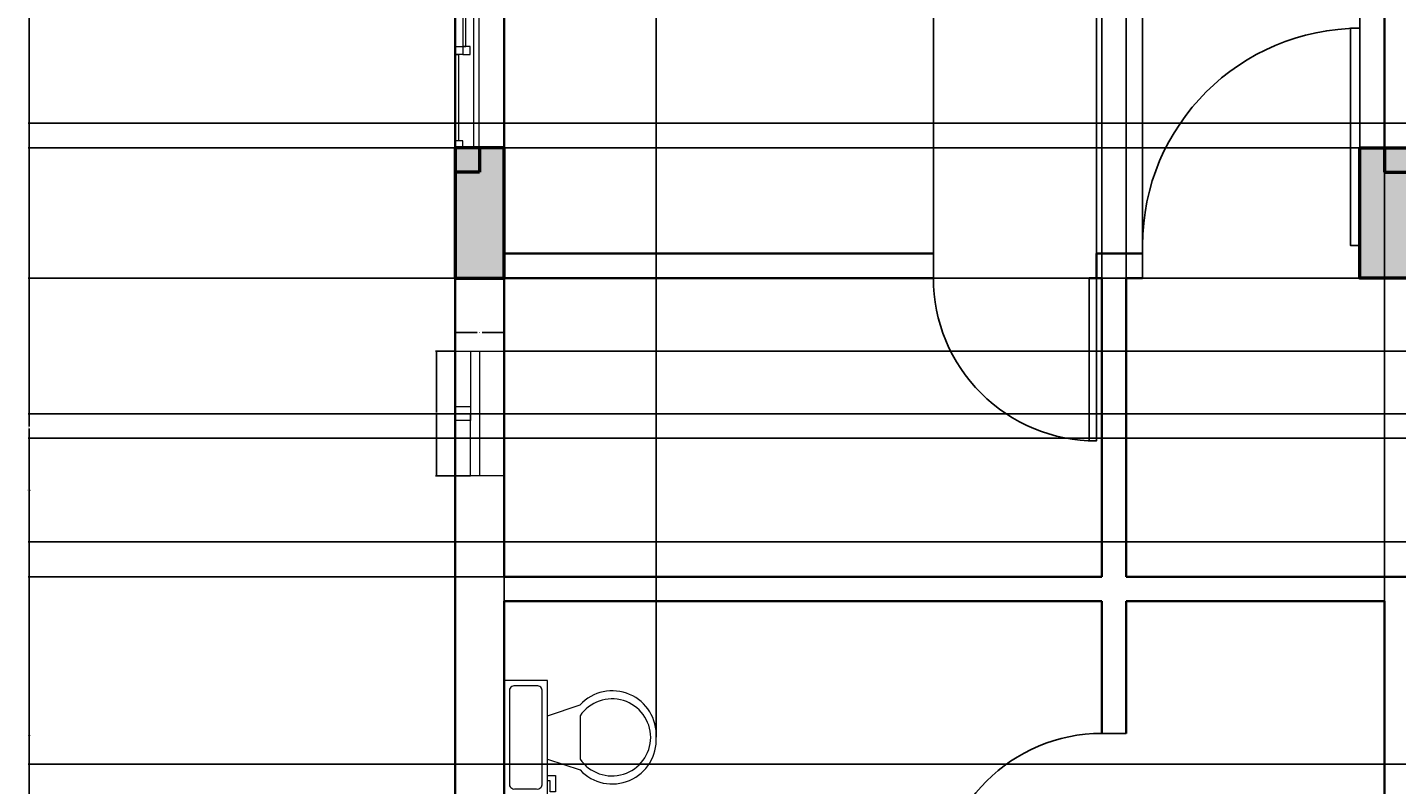
# Model space of a CAD drawing. Units: inches. Extents: x 393 to 993, y 153 to 660.
# Tile 2 of 6: x 393 to 645, y 359 to 499. Entities that reach past the tile are written whole.
import ezdxf

# ---------------------------------------------------------------- set-up
doc = ezdxf.new("R2010")
doc.units = ezdxf.units.IN
doc.header["$MEASUREMENT"] = 0
for name, color, linetype, lineweight in [('A-ANNO-DIMS', 2, 'Continuous', 18), ('A-COLS', 40, 'Continuous', 50), ('A-FLOR-FIXT', 9, 'Continuous', 18), ('A-GLAZ', 4, 'Continuous', 20), ('A-WALL', 40, 'Continuous', 35), ('DOORS', 32, 'Continuous', 25)]:
    doc.layers.add(name, color=color, linetype=linetype, lineweight=lineweight)
doc.styles.get("Standard").update_dxf_attribs({"font": 'arial.ttf'})
doc.dimstyles.get("Standard").update_dxf_attribs({"dimtxt": 0.18, "dimasz": 0.18, "dimexe": 0.18, "dimexo": 0.0625, "dimgap": 0.09, "dimtad": 0, "dimtih": 1, "dimtoh": 1, "dimdec": 1, "dimzin": 0, "dimdsep": 46, "dimlunit": 3, "dimtxsty": 'Standard', "dimcen": 0.09, "dimadec": 0, "dimazin": 0, "dimtfac": 1, "dimtdec": 1, "dimtofl": 0, "dimtmove": 0, "dimatfit": 3, "dimfxl": 1, "dimtolj": 1, "dimtzin": 0, "dimarcsym": 0})

# ---------------------------------------------------------------- blocks, each defined once
blk = doc.blocks.new('W')
for p, q in [((518.15, 606.48), (554.15, 606.48)), ((518.15, 605.48), (554.15, 605.48))]:
    blk.add_line(p, q)
for points in [[(518.15, 609.91), (554.15, 609.91), (554.15, 600.91), (518.15, 600.91)], [(519.42, 609.91), (518.15, 609.91), (518.15, 608.51), (519.42, 608.51)], [(519.42, 609.91), (535.35, 609.91), (535.35, 609.3), (519.42, 609.3)], [(535.35, 609.91), (536.78, 609.91), (536.78, 608.51), (535.35, 608.51)], [(536.78, 608.51), (535.35, 608.51), (535.35, 607.12), (536.78, 607.12)], [(552.72, 608.51), (536.78, 608.51), (536.78, 607.91), (552.72, 607.91)], [(552.72, 608.51), (554.15, 608.51), (554.15, 607.12), (552.72, 607.12)]]:
    blk.add_lwpolyline(points, close=True)
blk = doc.blocks.new('*U3')
for p, q in [((0, 0), (0, -6)), ((40, 0), (40, -6))]:
    blk.add_line(p, q)
blk.add_lwpolyline([(0, 0), (0, 40), (1.75, 40), (1.75, 0)], close=True)
blk.add_arc((0, 0), 40, 0, 90)
blk = doc.blocks.new('MM')
blk.add_line((476.48, 438.96), (476.48, 415.96))
for points in [[(471.98, 438.96), (480.98, 438.96), (480.98, 415.96), (471.98, 415.96), (471.98, 438.96)], [(471.98, 427.46), (471.98, 438.96), (474.84, 438.96), (474.84, 427.46)], [(471.98, 427.46), (471.98, 415.96), (474.84, 415.96), (474.84, 427.46)]]:
    blk.add_lwpolyline(points)
blk.add_lwpolyline([(471.98, 428.78), (474.84, 428.78), (474.84, 426.2), (471.98, 426.2)], close=True)
blk = doc.blocks.new('*U11')
for p, q in [((9.5, -6), (9.5, -2)), ((-10, -8.5), (-8, -8.5)), ((-10, -9.5), (-10, -8.5)), ((-7, -9.5), (-10, -9.5)), ((-8, -8.5), (-8, -8)), ((-7, -8), (-7, -9.5)), ((-4, -8), (-6, -14)), ((4, -8), (6, -14)), ((4, -14), (-4, -14))]:
    blk.add_line(p, q)
blk.add_lwpolyline([(10.5, -8), (10.5, 0), (-10.5, 0), (-10.5, -8)], close=True)
for points in [[(-9.5, -2), (-9.5, -6)], [(8.5, -1), (-8.5, -1)], [(-8.5, -7), (8.5, -7)]]:
    blk.add_lwpolyline(points)
for centre, radius, start, end in [((-8.625, -1.875), 0.8839, 81.8699, 188.1301), ((8.625, -1.875), 0.8839, 351.8699, 98.1301), ((-8.625, -6.125), 0.8839, 171.869898, 278.1301), ((8.625, -6.125), 0.8839, 261.8699, 8.1301), ((-0.4772, -19.9188), 8.0953, 133.01722, 273.38), ((0.0374, -19.8731), 7.127, 124.50543, 269.7), ((-0.0373, -19.8731), 7.127, 270.3, 55.4946), ((0.4773, -19.9188), 8.0953, 266.62, 46.9828)]:
    blk.add_arc(centre, radius, start, end)
blk = doc.blocks.new('COL-9X24-RH')
h = blk.add_hatch(color=256)
h.dxf.hatch_style = 1
h.paths.add_polyline_path([(4.5, 19.5), (4.5, 24), (0, 24), (0, 0), (9, 0), (9, 19.5)])
h = blk.add_hatch(color=256)
h.dxf.hatch_style = 1
h.paths.add_polyline_path([(4.5, 19.5), (9, 19.5), (9, 24), (4.5, 24)])
for p, q in [((4.5, 24), (4.5, 19.5)), ((4.5, 24), (9, 24)), ((9, 24), (9, 19.5)), ((4.5, 19.5), (9, 19.5))]:
    blk.add_line(p, q)
blk.add_lwpolyline([(0, 24), (9, 24), (9, 0), (0, 0), (0, 24)])
blk = doc.blocks.new('COL-9X24-LH')
h = blk.add_hatch(color=256)
h.dxf.hatch_style = 1
h.paths.add_polyline_path([(4.5, 24), (0, 24), (0, 19.5), (4.5, 19.5)])
h = blk.add_hatch(color=256)
h.dxf.hatch_style = 1
h.paths.add_polyline_path([(4.5, 19.5), (0, 19.5), (0, 0), (9, 0), (9, 24), (4.5, 24)])
for p, q in [((4.5, 24), (0, 24)), ((0, 24), (0, 19.5)), ((4.5, 24), (4.5, 19.5)), ((4.5, 19.5), (0, 19.5))]:
    blk.add_line(p, q)
blk.add_lwpolyline([(9, 24), (0, 24), (0, 0), (9, 0), (9, 24)])
blk = doc.blocks.new('*D26')
at = {"layer": 'A-ANNO-DIMS', "color": 0, "lineweight": -2, "transparency": 16777216}
for p, q in [((471.92, 438.96), (468.35, 438.96)), ((468.53, 438.78), (468.53, 427.64)), ((468.53, 416.14), (468.53, 427.27)), ((471.92, 415.96), (468.35, 415.96))]:
    blk.add_line(p, q, dxfattribs=at)
at = {"layer": 'A-ANNO-DIMS', "color": 0, "transparency": 16777216}
for points in [[(468.5, 438.78), (468.56, 438.78), (468.53, 438.96)], [(468.5, 416.14), (468.56, 416.14), (468.53, 415.96)]]:
    blk.add_solid(points, dxfattribs=at)
at = {"layer": 'Defpoints', "color": 0, "transparency": 16777216}
for p in [(468.53, 438.96), (471.98, 438.96), (471.98, 415.96)]:
    blk.add_point(p, dxfattribs=at)
at = {"layer": 'A-ANNO-DIMS', "color": 0, "transparency": 16777216, "insert": (468.53, 427.46), "char_height": 0.18, "attachment_point": 5}
blk.add_mtext('\\A1;WINDOW B 23 TYP.', dxfattribs=at)
blk = doc.blocks.new('*D27')
at = {"layer": 'A-ANNO-DIMS', "color": 0, "lineweight": -2, "transparency": 16777216}
for p, q in [((471.98, 439.02), (471.98, 442.59)), ((472.16, 442.41), (476.02, 442.41)), ((480.8, 442.41), (476.94, 442.41)), ((480.98, 439.02), (480.98, 442.59))]:
    blk.add_line(p, q, dxfattribs=at)
at = {"layer": 'A-ANNO-DIMS', "color": 0, "transparency": 16777216}
for points in [[(472.16, 442.44), (472.16, 442.38), (471.98, 442.41)], [(480.8, 442.44), (480.8, 442.38), (480.98, 442.41)]]:
    blk.add_solid(points, dxfattribs=at)
at = {"layer": 'Defpoints', "color": 0, "transparency": 16777216}
for p in [(480.98, 442.41), (471.98, 438.96), (480.98, 438.96)]:
    blk.add_point(p, dxfattribs=at)
at = {"layer": 'A-ANNO-DIMS', "color": 0, "transparency": 16777216, "insert": (476.48, 442.41), "char_height": 0.18, "attachment_point": 5}
blk.add_mtext('\\A1;9 TYP.', dxfattribs=at)
blk = doc.blocks.new('*D52')
at = {"layer": 'A-ANNO-DIMS', "color": 0, "lineweight": -2, "transparency": 16777216}
for p, q in [((480.92, 397.41), (393.4, 397.41)), ((393.58, 397.23), (393.58, 368.34)), ((393.58, 339.09), (393.58, 367.97)), ((471.92, 338.91), (393.4, 338.91))]:
    blk.add_line(p, q, dxfattribs=at)
at = {"layer": 'A-ANNO-DIMS', "color": 0, "transparency": 16777216}
for points in [[(393.55, 397.23), (393.61, 397.23), (393.58, 397.41)], [(393.55, 339.09), (393.61, 339.09), (393.58, 338.91)]]:
    blk.add_solid(points, dxfattribs=at)
at = {"layer": 'Defpoints', "color": 0, "transparency": 16777216}
for p in [(393.58, 397.41), (480.98, 397.41), (471.98, 338.91)]:
    blk.add_point(p, dxfattribs=at)
at = {"layer": 'A-ANNO-DIMS', "color": 0, "transparency": 16777216, "insert": (393.58, 368.16), "char_height": 0.18, "attachment_point": 5}
blk.add_mtext('\\A1;58.5', dxfattribs=at)
blk = doc.blocks.new('*D53')
at = {"layer": 'A-ANNO-DIMS', "color": 0, "lineweight": -2, "transparency": 16777216}
for p, q in [((471.92, 452.41), (393.4, 452.41)), ((393.58, 452.23), (393.58, 425.09)), ((393.58, 397.59), (393.58, 424.73)), ((480.92, 397.41), (393.4, 397.41))]:
    blk.add_line(p, q, dxfattribs=at)
at = {"layer": 'A-ANNO-DIMS', "color": 0, "transparency": 16777216}
for points in [[(393.55, 452.23), (393.61, 452.23), (393.58, 452.41)], [(393.55, 397.59), (393.61, 397.59), (393.58, 397.41)]]:
    blk.add_solid(points, dxfattribs=at)
at = {"layer": 'Defpoints', "color": 0, "transparency": 16777216}
for p in [(393.58, 452.41), (471.98, 452.41), (480.98, 397.41)]:
    blk.add_point(p, dxfattribs=at)
at = {"layer": 'A-ANNO-DIMS', "color": 0, "transparency": 16777216, "insert": (393.58, 424.91), "char_height": 0.18, "attachment_point": 5}
blk.add_mtext('\\A1;55', dxfattribs=at)
blk = doc.blocks.new('*D54')
at = {"layer": 'A-ANNO-DIMS', "color": 0, "lineweight": -2, "transparency": 16777216}
for p, q in [((471.92, 609.91), (393.4, 609.91)), ((393.58, 609.73), (393.58, 531.34)), ((393.58, 452.59), (393.58, 530.97)), ((471.92, 452.41), (393.4, 452.41))]:
    blk.add_line(p, q, dxfattribs=at)
at = {"layer": 'A-ANNO-DIMS', "color": 0, "transparency": 16777216}
for points in [[(393.55, 609.73), (393.61, 609.73), (393.58, 609.91)], [(393.55, 452.59), (393.61, 452.59), (393.58, 452.41)]]:
    blk.add_solid(points, dxfattribs=at)
at = {"layer": 'Defpoints', "color": 0, "transparency": 16777216}
for p in [(393.58, 609.91), (471.98, 609.91), (471.98, 452.41)]:
    blk.add_point(p, dxfattribs=at)
at = {"layer": 'A-ANNO-DIMS', "color": 0, "transparency": 16777216, "insert": (393.58, 531.16), "char_height": 0.18, "attachment_point": 5}
blk.add_mtext('\\A1;157.5', dxfattribs=at)
blk = doc.blocks.new('*D56')
at = {"layer": 'A-ANNO-DIMS', "color": 0, "lineweight": -2, "transparency": 16777216}
for p, q in [((480.98, 397.47), (480.98, 660.49)), ((481.16, 660.31), (535.7, 660.31)), ((590.8, 660.31), (536.26, 660.31)), ((590.98, 397.47), (590.98, 660.49))]:
    blk.add_line(p, q, dxfattribs=at)
at = {"layer": 'A-ANNO-DIMS', "color": 0, "transparency": 16777216}
for points in [[(481.16, 660.34), (481.16, 660.28), (480.98, 660.31)], [(590.8, 660.34), (590.8, 660.28), (590.98, 660.31)]]:
    blk.add_solid(points, dxfattribs=at)
at = {"layer": 'Defpoints', "color": 0, "transparency": 16777216}
for p in [(590.98, 660.31), (480.98, 397.41), (590.98, 397.41)]:
    blk.add_point(p, dxfattribs=at)
at = {"layer": 'A-ANNO-DIMS', "color": 0, "transparency": 16777216, "insert": (535.98, 660.31), "char_height": 0.18, "attachment_point": 5}
blk.add_mtext('\\A1;110', dxfattribs=at)
blk = doc.blocks.new('*D61')
at = {"layer": 'A-ANNO-DIMS', "color": 0, "lineweight": -2, "transparency": 16777216}
for p, q in [((559.98, 452.47), (559.98, 660.49)), ((560.16, 660.31), (574.76, 660.31)), ((589.8, 660.31), (575.2, 660.31)), ((589.98, 452.47), (589.98, 660.49))]:
    blk.add_line(p, q, dxfattribs=at)
at = {"layer": 'A-ANNO-DIMS', "color": 0, "transparency": 16777216}
for points in [[(560.16, 660.34), (560.16, 660.28), (559.98, 660.31)], [(589.8, 660.34), (589.8, 660.28), (589.98, 660.31)]]:
    blk.add_solid(points, dxfattribs=at)
at = {"layer": 'Defpoints', "color": 0, "transparency": 16777216}
for p in [(589.98, 660.31), (559.98, 452.41), (589.98, 452.41)]:
    blk.add_point(p, dxfattribs=at)
at = {"layer": 'A-ANNO-DIMS', "color": 0, "transparency": 16777216, "insert": (574.98, 660.31), "char_height": 0.18, "attachment_point": 5}
blk.add_mtext('\\A1;30', dxfattribs=at)
blk = doc.blocks.new('*D62')
at = {"layer": 'A-ANNO-DIMS', "color": 0, "lineweight": -2, "transparency": 16777216}
for p, q in [((848.42, 422.91), (393.4, 422.91)), ((393.58, 422.73), (393.58, 393.09)), ((393.58, 363.09), (393.58, 392.72)), ((848.42, 362.91), (393.4, 362.91))]:
    blk.add_line(p, q, dxfattribs=at)
at = {"layer": 'A-ANNO-DIMS', "color": 0, "transparency": 16777216}
for points in [[(393.55, 422.73), (393.61, 422.73), (393.58, 422.91)], [(393.55, 363.09), (393.61, 363.09), (393.58, 362.91)]]:
    blk.add_solid(points, dxfattribs=at)
at = {"layer": 'Defpoints', "color": 0, "transparency": 16777216}
for p in [(393.58, 422.91), (848.48, 422.91), (848.48, 362.91)]:
    blk.add_point(p, dxfattribs=at)
at = {"layer": 'A-ANNO-DIMS', "color": 0, "transparency": 16777216, "insert": (393.58, 392.91), "char_height": 0.18, "attachment_point": 5}
blk.add_mtext('\\A1;60', dxfattribs=at)
blk = doc.blocks.new('*D63')
at = {"layer": 'A-ANNO-DIMS', "color": 0, "lineweight": -2, "transparency": 16777216}
for p, q in [((960.92, 476.41), (393.4, 476.41)), ((393.58, 476.23), (393.58, 452.09)), ((393.58, 427.59), (393.58, 451.72)), ((960.92, 427.41), (393.4, 427.41))]:
    blk.add_line(p, q, dxfattribs=at)
at = {"layer": 'A-ANNO-DIMS', "color": 0, "transparency": 16777216}
for points in [[(393.55, 476.23), (393.61, 476.23), (393.58, 476.41)], [(393.55, 427.59), (393.61, 427.59), (393.58, 427.41)]]:
    blk.add_solid(points, dxfattribs=at)
at = {"layer": 'Defpoints', "color": 0, "transparency": 16777216}
for p in [(393.58, 476.41), (960.98, 476.41), (960.98, 427.41)]:
    blk.add_point(p, dxfattribs=at)
at = {"layer": 'A-ANNO-DIMS', "color": 0, "transparency": 16777216, "insert": (393.58, 451.91), "char_height": 0.18, "attachment_point": 5}
blk.add_mtext('\\A1;49', dxfattribs=at)
blk = doc.blocks.new('*D64')
at = {"layer": 'A-ANNO-DIMS', "color": 0, "lineweight": -2, "transparency": 16777216}
for p, q in [((932.42, 576.91), (393.4, 576.91)), ((393.58, 576.73), (393.58, 529.09)), ((393.58, 481.09), (393.58, 528.72)), ((932.42, 480.91), (393.4, 480.91))]:
    blk.add_line(p, q, dxfattribs=at)
at = {"layer": 'A-ANNO-DIMS', "color": 0, "transparency": 16777216}
for points in [[(393.55, 576.73), (393.61, 576.73), (393.58, 576.91)], [(393.55, 481.09), (393.61, 481.09), (393.58, 480.91)]]:
    blk.add_solid(points, dxfattribs=at)
at = {"layer": 'Defpoints', "color": 0, "transparency": 16777216}
for p in [(393.58, 576.91), (932.48, 576.91), (932.48, 480.91)]:
    blk.add_point(p, dxfattribs=at)
at = {"layer": 'A-ANNO-DIMS', "color": 0, "transparency": 16777216, "insert": (393.58, 528.91), "char_height": 0.18, "attachment_point": 5}
blk.add_mtext('\\A1;96', dxfattribs=at)
blk = doc.blocks.new('*D65')
at = {"layer": 'A-ANNO-DIMS', "color": 0, "lineweight": -2, "transparency": 16777216}
for p, q in [((598.48, 456.97), (598.48, 660.49)), ((598.66, 660.31), (618.26, 660.31)), ((638.3, 660.31), (618.7, 660.31)), ((638.48, 458.47), (638.48, 660.49))]:
    blk.add_line(p, q, dxfattribs=at)
at = {"layer": 'A-ANNO-DIMS', "color": 0, "transparency": 16777216}
for points in [[(598.66, 660.34), (598.66, 660.28), (598.48, 660.31)], [(638.3, 660.34), (638.3, 660.28), (638.48, 660.31)]]:
    blk.add_solid(points, dxfattribs=at)
at = {"layer": 'Defpoints', "color": 0, "transparency": 16777216}
for p in [(638.48, 660.31), (598.48, 456.91), (638.48, 458.41)]:
    blk.add_point(p, dxfattribs=at)
at = {"layer": 'A-ANNO-DIMS', "color": 0, "transparency": 16777216, "insert": (618.48, 660.31), "char_height": 0.18, "attachment_point": 5}
blk.add_mtext('\\A1;40', dxfattribs=at)
blk = doc.blocks.new('*D72')
at = {"layer": 'A-ANNO-DIMS', "color": 0, "lineweight": -2, "transparency": 16777216}
for p, q in [((481.04, 452.41), (993.06, 452.41)), ((992.88, 452.23), (992.88, 445.86)), ((992.88, 439.14), (992.88, 445.5)), ((481.04, 438.96), (993.06, 438.96))]:
    blk.add_line(p, q, dxfattribs=at)
at = {"layer": 'A-ANNO-DIMS', "color": 0, "transparency": 16777216}
for points in [[(992.85, 452.23), (992.91, 452.23), (992.88, 452.41)], [(992.85, 439.14), (992.91, 439.14), (992.88, 438.96)]]:
    blk.add_solid(points, dxfattribs=at)
at = {"layer": 'Defpoints', "color": 0, "transparency": 16777216}
for p in [(480.98, 452.41), (992.88, 452.41), (480.98, 438.96)]:
    blk.add_point(p, dxfattribs=at)
at = {"layer": 'A-ANNO-DIMS', "color": 0, "transparency": 16777216, "insert": (992.88, 445.68), "char_height": 0.18, "attachment_point": 5}
blk.add_mtext('\\A1;13.45', dxfattribs=at)
blk = doc.blocks.new('*D73')
at = {"layer": 'A-ANNO-DIMS', "color": 0, "lineweight": -2, "transparency": 16777216}
for p, q in [((956.42, 422.91), (393.4, 422.91)), ((393.58, 422.73), (393.58, 413.55)), ((393.58, 404.01), (393.58, 413.19)), ((956.42, 403.83), (393.4, 403.83))]:
    blk.add_line(p, q, dxfattribs=at)
at = {"layer": 'A-ANNO-DIMS', "color": 0, "transparency": 16777216}
for points in [[(393.55, 422.73), (393.61, 422.73), (393.58, 422.91)], [(393.55, 404.01), (393.61, 404.01), (393.58, 403.83)]]:
    blk.add_solid(points, dxfattribs=at)
at = {"layer": 'Defpoints', "color": 0, "transparency": 16777216}
for p in [(393.58, 422.91), (956.48, 422.91), (956.48, 403.83)]:
    blk.add_point(p, dxfattribs=at)
at = {"layer": 'A-ANNO-DIMS', "color": 0, "transparency": 16777216, "insert": (393.58, 413.37), "char_height": 0.18, "attachment_point": 5}
blk.add_mtext('\\A1;19.08', dxfattribs=at)
blk = doc.blocks.new('*D77')
at = {"layer": 'A-ANNO-DIMS', "color": 0, "lineweight": -2, "transparency": 16777216}
for p, q in [((595.48, 397.47), (595.48, 660.49)), ((595.66, 660.31), (618.9, 660.31)), ((642.8, 660.31), (619.56, 660.31)), ((642.98, 392.97), (642.98, 660.49))]:
    blk.add_line(p, q, dxfattribs=at)
at = {"layer": 'A-ANNO-DIMS', "color": 0, "transparency": 16777216}
for points in [[(595.66, 660.34), (595.66, 660.28), (595.48, 660.31)], [(642.8, 660.34), (642.8, 660.28), (642.98, 660.31)]]:
    blk.add_solid(points, dxfattribs=at)
at = {"layer": 'Defpoints', "color": 0, "transparency": 16777216}
for p in [(642.98, 660.31), (595.48, 397.41), (642.98, 392.91)]:
    blk.add_point(p, dxfattribs=at)
at = {"layer": 'A-ANNO-DIMS', "color": 0, "transparency": 16777216, "insert": (619.23, 660.31), "char_height": 0.18, "attachment_point": 5}
blk.add_mtext('\\A1;47.5', dxfattribs=at)
blk = doc.blocks.new('*D79')
at = {"layer": 'A-ANNO-DIMS', "color": 0, "lineweight": -2, "transparency": 16777216}
for p, q in [((480.98, 378.39), (480.98, 660.49)), ((481.16, 660.31), (494.76, 660.31)), ((508.8, 660.31), (495.2, 660.31)), ((508.98, 367.89), (508.98, 660.49))]:
    blk.add_line(p, q, dxfattribs=at)
at = {"layer": 'A-ANNO-DIMS', "color": 0, "transparency": 16777216}
for points in [[(481.16, 660.34), (481.16, 660.28), (480.98, 660.31)], [(508.8, 660.34), (508.8, 660.28), (508.98, 660.31)]]:
    blk.add_solid(points, dxfattribs=at)
at = {"layer": 'Defpoints', "color": 0, "transparency": 16777216}
for p in [(508.98, 660.31), (480.98, 378.32), (508.98, 367.82)]:
    blk.add_point(p, dxfattribs=at)
at = {"layer": 'A-ANNO-DIMS', "color": 0, "transparency": 16777216, "insert": (494.98, 660.31), "char_height": 0.18, "attachment_point": 5}
blk.add_mtext('\\A1;28', dxfattribs=at)
blk = doc.blocks.new('*D80')
at = {"layer": 'A-ANNO-DIMS', "color": 0, "lineweight": -2, "transparency": 16777216}
for p, q in [((879.42, 480.91), (393.4, 480.91)), ((393.58, 480.73), (393.58, 478.84)), ((879.42, 476.41), (393.4, 476.41)), ((393.58, 476.59), (393.58, 478.48))]:
    blk.add_line(p, q, dxfattribs=at)
at = {"layer": 'A-ANNO-DIMS', "color": 0, "transparency": 16777216}
for points in [[(393.55, 480.73), (393.61, 480.73), (393.58, 480.91)], [(393.55, 476.59), (393.61, 476.59), (393.58, 476.41)]]:
    blk.add_solid(points, dxfattribs=at)
at = {"layer": 'Defpoints', "color": 0, "transparency": 16777216}
for p in [(393.58, 480.91), (879.48, 480.91), (879.48, 476.41)]:
    blk.add_point(p, dxfattribs=at)
at = {"layer": 'A-ANNO-DIMS', "color": 0, "transparency": 16777216, "insert": (393.58, 478.66), "char_height": 0.18, "attachment_point": 5}
blk.add_mtext('\\A1;4.5', dxfattribs=at)

msp = doc.modelspace()

# ---------------------------------------------------------------- linework, layer by layer
at = {"layer": 'A-WALL'}
for p, q in [((471.9798, 609.9066), (471.9798, 180.9066)), ((480.9798, 600.9066), (480.9798, 456.9066)), ((642.9798, 600.9066), (642.9798, 476.4066)), ((480.9798, 456.9066), (559.9798, 456.9066)), ((589.9798, 452.4066), (589.9798, 456.9066)), ((589.9798, 456.9066), (598.4798, 456.9066)), ((480.9798, 452.4066), (559.9798, 452.4066)), ((480.9798, 452.4066), (480.9798, 397.4066)), ((588.6673, 452.4066), (590.9798, 452.4066)), ((590.9798, 452.4066), (589.9798, 452.4066)), ((590.9798, 452.4066), (590.9798, 397.4066)), ((595.4798, 452.4066), (595.4798, 397.4066)), ((595.4798, 452.4066), (598.4798, 452.4066)), ((480.9798, 397.4066), (590.9798, 397.4066)), ((595.4798, 397.4066), (642.9798, 397.4066)), ((642.9798, 397.4066), (647.4798, 397.4066)), ((480.9798, 392.9066), (590.9798, 392.9066)), ((480.9798, 392.9066), (480.9798, 180.9066)), ((590.9798, 392.9066), (590.9798, 368.5513)), ((595.4798, 392.9066), (642.9798, 392.9066)), ((595.4798, 392.9066), (595.4798, 368.5513)), ((642.9798, 392.9066), (641.9798, 392.9066)), ((642.9798, 392.9066), (642.9798, 314.9066))]:
    msp.add_line(p, q, dxfattribs=at)

# ---------------------------------------------------------------- block references
at = {"layer": 'A-COLS'}
for name, p in [('COL-9X24-LH', (471.98, 452.407)), ('COL-9X24-RH', (638.48, 452.407))]:
    msp.add_blockref(name, p, dxfattribs=at)
at = {"layer": 'A-FLOR-FIXT', "rotation": 90}
msp.add_blockref('*U11', (480.9798, 367.8225), dxfattribs=at)
at = {"layer": 'A-GLAZ', "rotation": 90}
msp.add_blockref('W', (1081.8865, -41.7421), dxfattribs=at)
at = {"layer": 'A-GLAZ'}
msp.add_blockref('MM', (0, 0), dxfattribs=at)
at = {"layer": 'DOORS', "xscale": -1}
msp.add_blockref('*U3', (638.4798, 458.4066), dxfattribs=at)
at = {"layer": 'DOORS', "xscale": 0.75, "yscale": 0.75, "zscale": 0.75}
for p, rotation in [((589.9798, 452.4066), 180.0000000000003), ((590.9798, 338.5513), 90.00000000000031)]:
    msp.add_blockref('*U3', p, dxfattribs=dict(at, rotation=rotation))

# ---------------------------------------------------------------- dimensions: what is measured, and where the dimension line sits
at = {"layer": 'A-ANNO-DIMS'}
for base, p1, p2, override, picture, middle in [((590.9798, 660.3066), (480.9798, 397.4066), (590.9798, 397.4066), {"dimdec": 0, "dimlfac": 1, "dimrnd": 0, "dimzin": 0, "dimdsep": 46, "dimlunit": 2}, '*D56', (535.9798, 660.3066)), ((508.9798, 660.3066), (480.9798, 378.3225), (508.9798, 367.8226), {"dimdec": 0, "dimlfac": 1, "dimrnd": 0, "dimzin": 0, "dimdsep": 46, "dimlunit": 2}, '*D79', (494.9798, 660.3066)), ((589.9798, 660.3066), (559.9798, 452.4066), (589.9798, 452.4066), {"dimdec": 0, "dimlfac": 1, "dimrnd": 0, "dimzin": 0, "dimdsep": 46, "dimlunit": 2}, '*D61', (574.9798, 660.3066)), ((642.9798, 660.3066), (595.4798, 397.4066), (642.9798, 392.9066), {"dimdec": 1, "dimlfac": 1, "dimrnd": 0, "dimzin": 0, "dimdsep": 46, "dimlunit": 2}, '*D77', (619.2298, 660.3066)), ((638.4798, 660.3066), (598.4798, 456.9066), (638.4798, 458.4066), {"dimdec": 0, "dimlfac": 1, "dimrnd": 0, "dimzin": 0, "dimdsep": 46, "dimlunit": 2}, '*D65', (618.4798, 660.3066))]:
    dim = msp.add_linear_dim(base=base, p1=p1, p2=p2, dimstyle='Standard', override=override, dxfattribs=at)
    dim.commit()
    dim.dimension.update_dxf_attribs({"geometry": picture, "text_midpoint": middle})
for base, p1, p2, override, picture, middle in [((393.5798, 609.9066), (471.9798, 452.4066), (471.9798, 609.9066), {"dimdec": 1, "dimlfac": 1, "dimrnd": 0, "dimzin": 0, "dimdsep": 46, "dimlunit": 2}, '*D54', (393.5798, 531.1566)), ((393.5798, 576.9066), (932.4798, 480.9066), (932.4798, 576.9066), {"dimdec": 0, "dimlfac": 1, "dimrnd": 0, "dimzin": 0, "dimdsep": 46, "dimlunit": 2}, '*D64', (393.5798, 528.9066)), ((393.5798, 480.9066), (879.4798, 476.4066), (879.4798, 480.9066), {"dimdec": 1, "dimlfac": 1, "dimrnd": 0, "dimzin": 0, "dimdsep": 46, "dimlunit": 2}, '*D80', (393.5798, 478.6566)), ((393.5798, 476.4066), (960.9798, 427.4066), (960.9798, 476.4066), {"dimdec": 0, "dimlfac": 1, "dimrnd": 0, "dimzin": 0, "dimdsep": 46, "dimlunit": 2}, '*D63', (393.5798, 451.9066)), ((393.5798, 452.4066), (480.9798, 397.4066), (471.9798, 452.4066), {"dimdec": 0, "dimlfac": 1, "dimrnd": 0, "dimzin": 0, "dimdsep": 46, "dimlunit": 2}, '*D53', (393.5798, 424.9066)), ((992.8798, 452.4066), (480.9798, 438.9566), (480.9798, 452.4066), {"dimdec": 2, "dimlfac": 1, "dimrnd": 0, "dimzin": 0, "dimdsep": 46, "dimlunit": 2}, '*D72', (992.8798, 445.6816)), ((393.5798, 422.9066), (956.4798, 403.8282), (956.4798, 422.9066), {"dimdec": 2, "dimlfac": 1, "dimrnd": 0, "dimzin": 0, "dimdsep": 46, "dimlunit": 2}, '*D73', (393.5798, 413.3674)), ((393.5798, 422.9066), (848.4798, 362.9066), (848.4798, 422.9066), {"dimdec": 0, "dimlfac": 1, "dimrnd": 0, "dimzin": 0, "dimdsep": 46, "dimlunit": 2}, '*D62', (393.5798, 392.9066)), ((393.5798, 397.4066), (471.9798, 338.9066), (480.9798, 397.4066), {"dimdec": 1, "dimlfac": 1, "dimrnd": 0, "dimzin": 0, "dimdsep": 46, "dimlunit": 2}, '*D52', (393.5798, 368.1566))]:
    dim = msp.add_linear_dim(base=base, p1=p1, p2=p2, angle=90, dimstyle='Standard', override=override, dxfattribs=at)
    dim.commit()
    dim.dimension.update_dxf_attribs({"geometry": picture, "text_midpoint": middle})
dim = msp.add_linear_dim(base=(480.9798, 442.4066), p1=(471.9798, 438.9566), p2=(480.9798, 438.9566), text='<> TYP.', dimstyle='Standard', override={"dimdec": 0, "dimlfac": 1, "dimrnd": 0, "dimzin": 0, "dimdsep": 46, "dimlunit": 2}, dxfattribs=at)
dim.commit()
dim.dimension.update_dxf_attribs({"geometry": '*D27', "text_midpoint": (476.4798, 442.4066)})
dim = msp.add_linear_dim(base=(468.5298, 438.9566), p1=(471.9798, 415.9566), p2=(471.9798, 438.9566), angle=90, text='WINDOW B <> TYP.', dimstyle='Standard', override={"dimdec": 0, "dimlfac": 1, "dimrnd": 0, "dimzin": 0, "dimdsep": 46, "dimlunit": 2}, dxfattribs=at)
dim.commit()
dim.dimension.update_dxf_attribs({"geometry": '*D26', "text_midpoint": (468.5298, 427.4566)})

doc.saveas('drawing.dxf')
